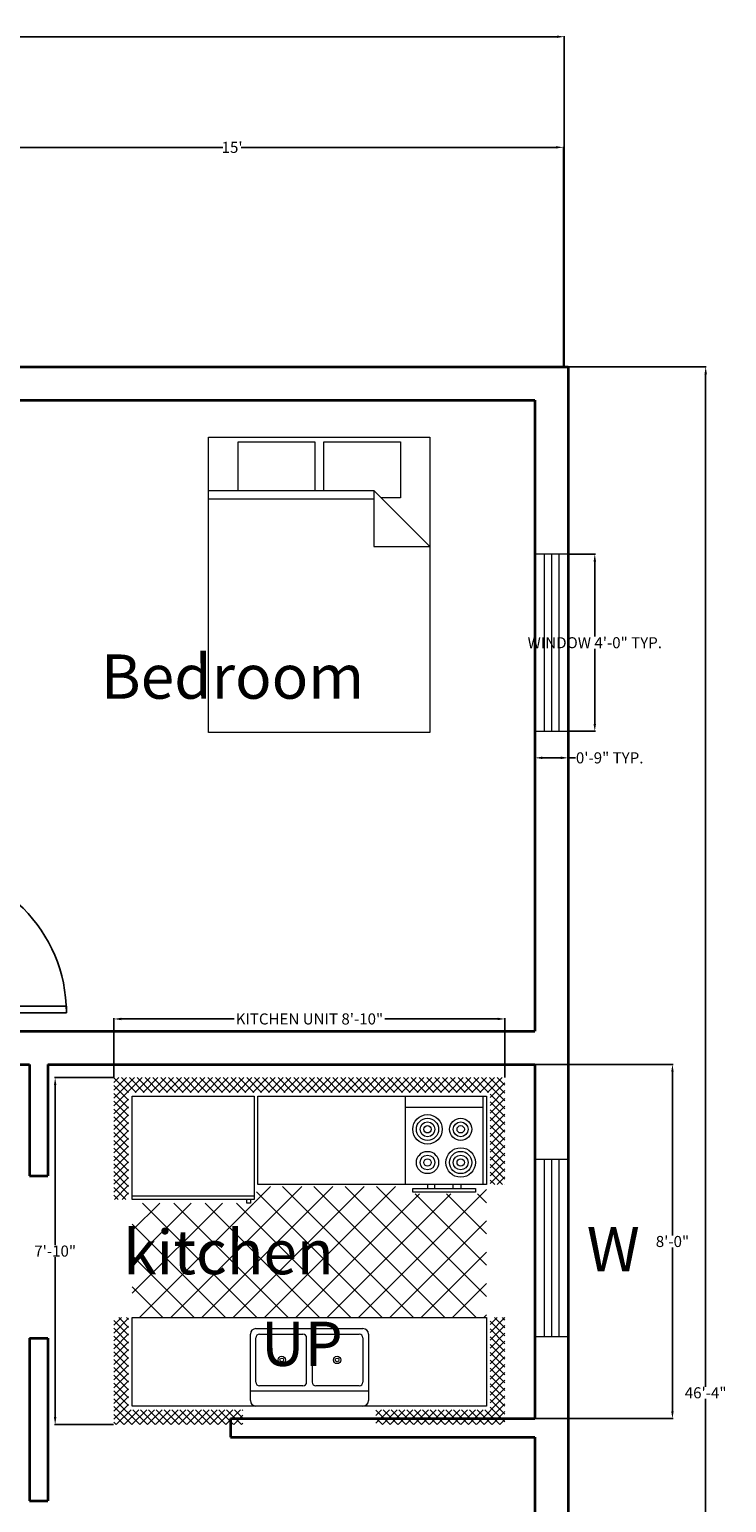
# Model space of a CAD drawing. Units: inches. Extents: x 751 to 1500, y 610 to 1297.
# Tile 4 of 4: x 1308 to 1497, y 898 to 1297. Entities that reach past the tile are written whole.
import ezdxf

# ---------------------------------------------------------------- set-up
doc = ezdxf.new("R2010")
doc.units = ezdxf.units.IN
doc.header["$MEASUREMENT"] = 0
doc.layers.get('0').update_dxf_attribs({"color": 1})
for name, color, linetype, lineweight in [('A-ANNO-DIMS', 5, 'Continuous', 18), ('A-ANNO-TEXT', 7, 'Continuous', 18), ('A-AREA-IDEN', 7, 'Continuous', 25), ('A-FLOR-FIXT', 9, 'Continuous', 18), ('A-FURN', 8, 'Continuous', 18), ('door', 2, 'Continuous', 25), ('wall', 6, 'Continuous', 35), ('windows', 70, 'Continuous', 18)]:
    doc.layers.add(name, color=color, linetype=linetype, lineweight=lineweight)
doc.styles.get("Standard").update_dxf_attribs({"font": 'arial.ttf'})
doc.dimstyles.get("Standard").update_dxf_attribs({"dimtxt": 3, "dimasz": 2, "dimexe": 0.18, "dimexo": 0.0625, "dimgap": 0.09, "dimtad": 0, "dimtih": 1, "dimtoh": 1, "dimdec": 0, "dimzin": 0, "dimdsep": 46, "dimlunit": 3, "dimtxsty": 'Standard', "dimcen": 0.09, "dimadec": 0, "dimazin": 0, "dimtfac": 1, "dimtdec": 0, "dimtofl": 0, "dimtmove": 0, "dimatfit": 3, "dimfxl": 1, "dimtolj": 1, "dimtzin": 0, "dimarcsym": 0})

# ---------------------------------------------------------------- blocks, each defined once
blk = doc.blocks.new('*U3')
for p, q in [((0, 0), (0, 6)), ((40, 0), (40, 6))]:
    blk.add_line(p, q)
blk.add_lwpolyline([(0, 0), (0, -40), (1.75, -40), (1.75, 0)], close=True)
blk.add_arc((0, 0), 40, 270, 360)
blk = doc.blocks.new('*D8')
at = {"layer": 'A-ANNO-DIMS', "color": 0, "lineweight": -2, "transparency": 16777216}
for p, q in [((989.16, 1207.18), (989.16, 1295.32)), ((991.16, 1295.14), (1215.8, 1295.14)), ((1450.93, 1295.14), (1226.29, 1295.14)), ((1452.93, 1205.96), (1452.93, 1295.32))]:
    blk.add_line(p, q, dxfattribs=at)
at = {"layer": 'A-ANNO-DIMS', "color": 0, "transparency": 16777216}
for points in [[(991.16, 1295.48), (991.16, 1294.81), (989.16, 1295.14)], [(1450.93, 1295.48), (1450.93, 1294.81), (1452.93, 1295.14)]]:
    blk.add_solid(points, dxfattribs=at)
at = {"layer": 'Defpoints', "color": 0, "transparency": 16777216}
for p in [(1452.93, 1295.14), (989.16, 1207.12), (1452.93, 1205.9)]:
    blk.add_point(p, dxfattribs=at)
at = {"layer": 'A-ANNO-DIMS', "color": 0, "transparency": 16777216, "insert": (1221.05, 1295.14), "char_height": 3, "attachment_point": 5}
blk.add_mtext('\\A1;38\'-8"', dxfattribs=at)
blk = doc.blocks.new('*D11')
at = {"layer": 'A-ANNO-DIMS', "color": 0, "lineweight": -2, "transparency": 16777216}
for p, q in [((1273.13, 1207.41), (1273.13, 1265.35)), ((1452.66, 1205.46), (1452.66, 1265.35)), ((1275.13, 1265.17), (1360.4, 1265.17)), ((1450.66, 1265.17), (1365.39, 1265.17))]:
    blk.add_line(p, q, dxfattribs=at)
at = {"layer": 'A-ANNO-DIMS', "color": 0, "transparency": 16777216}
for points in [[(1275.13, 1265.51), (1275.13, 1264.84), (1273.13, 1265.17)], [(1450.66, 1265.51), (1450.66, 1264.84), (1452.66, 1265.17)]]:
    blk.add_solid(points, dxfattribs=at)
at = {"layer": 'Defpoints', "color": 0, "transparency": 16777216}
for p in [(1452.66, 1265.17), (1273.13, 1207.34), (1452.66, 1205.4)]:
    blk.add_point(p, dxfattribs=at)
at = {"layer": 'A-ANNO-DIMS', "color": 0, "transparency": 16777216, "insert": (1362.9, 1265.17), "char_height": 3, "attachment_point": 5}
blk.add_mtext("\\A1;15'", dxfattribs=at)
blk = doc.blocks.new('Kitchen Layout - 7 x 8 ft')
for p, q in [((-5, 81.32), (2.68, 89)), ((-5, 83.44), (0.56, 89)), ((-5, 85.56), (-1.56, 89)), ((-5, 87.68), (-3.68, 89)), ((-1, 84.97), (-5, 88.97)), ((1.09, 85), (-2.91, 89)), ((3.21, 85), (-0.79, 89)), ((0.81, 85), (4.81, 89)), ((5.34, 85), (1.34, 89)), ((2.93, 85), (6.93, 89)), ((7.46, 85), (3.46, 89)), ((5.05, 85), (9.05, 89)), ((9.58, 85), (5.58, 89)), ((7.17, 85), (11.17, 89)), ((11.7, 85), (7.7, 89)), ((9.29, 85), (13.29, 89)), ((13.82, 85), (9.82, 89)), ((11.41, 85), (15.41, 89)), ((15.94, 85), (11.94, 89)), ((13.53, 85), (17.53, 89)), ((18.06, 85), (14.06, 89)), ((15.65, 85), (19.65, 89)), ((20.18, 85), (16.18, 89)), ((17.78, 85), (21.78, 89)), ((22.31, 85), (18.31, 89)), ((19.9, 85), (23.9, 89)), ((24.43, 85), (20.43, 89)), ((22.02, 85), (26.02, 89)), ((26.55, 85), (22.55, 89)), ((24.14, 85), (28.14, 89)), ((28.67, 85), (24.67, 89)), ((26.26, 85), (30.26, 89)), ((30.79, 85), (26.79, 89)), ((28.38, 85), (32.38, 89)), ((32.91, 85), (28.91, 89)), ((30.5, 85), (34.5, 89)), ((35.03, 85), (31.03, 89)), ((32.63, 85), (36.63, 89)), ((37.16, 85), (33.16, 89)), ((34.75, 85), (38.75, 89)), ((39.28, 85), (35.28, 89)), ((36.87, 85), (40.87, 89)), ((41.4, 85), (37.4, 89)), ((38.99, 85), (42.99, 89)), ((43.52, 85), (39.52, 89)), ((41.11, 85), (45.11, 89)), ((45.64, 85), (41.64, 89)), ((43.23, 85), (47.23, 89)), ((47.76, 85), (43.76, 89)), ((45.35, 85), (49.35, 89)), ((49.88, 85), (45.88, 89)), ((47.47, 85), (51.47, 89)), ((52, 85), (48, 89)), ((49.6, 85), (53.6, 89)), ((54.13, 85), (50.13, 89)), ((51.72, 85), (55.72, 89)), ((56.25, 85), (52.25, 89)), ((53.84, 85), (57.84, 89)), ((58.37, 85), (54.37, 89)), ((55.96, 85), (59.96, 89)), ((60.49, 85), (56.49, 89)), ((58.08, 85), (62.08, 89)), ((62.61, 85), (58.61, 89)), ((60.2, 85), (64.2, 89)), ((64.73, 85), (60.73, 89)), ((62.32, 85), (66.32, 89)), ((66.85, 85), (62.85, 89)), ((64.45, 85), (68.45, 89)), ((68.97, 85), (64.97, 89)), ((66.57, 85), (70.57, 89)), ((71.1, 85), (67.1, 89)), ((68.69, 85), (72.69, 89)), ((73.22, 85), (69.22, 89)), ((70.81, 85), (74.81, 89)), ((75.34, 85), (71.34, 89)), ((72.93, 85), (76.93, 89)), ((77.46, 85), (73.46, 89)), ((75.05, 85), (79.05, 89)), ((79.58, 85), (75.58, 89)), ((77.17, 85), (81.17, 89)), ((81.7, 85), (77.7, 89)), ((79.29, 85), (83.29, 89)), ((83.82, 85), (79.82, 89)), ((81.42, 85), (85.42, 89)), ((85.95, 85), (81.95, 89)), ((83.54, 85), (87.54, 89)), ((88.07, 85), (84.07, 89)), ((85.66, 85), (89.66, 89)), ((90.19, 85), (86.19, 89)), ((87.78, 85), (91.78, 89)), ((92.31, 85), (88.31, 89)), ((89.9, 85), (93.9, 89)), ((94.43, 85), (90.43, 89)), ((92.02, 85), (96.02, 89)), ((96.55, 85), (92.55, 89)), ((94.14, 85), (98.14, 89)), ((101, 82.67), (94.67, 89)), ((96.27, 85), (100.27, 89)), ((101, 84.79), (96.79, 89)), ((101, 86.92), (98.92, 89)), ((-1, 82.85), (-5, 86.85)), ((-1, 80.73), (-5, 84.73)), ((34, 84), (96, 84)), ((34, 60), (34, 84)), ((96, 84), (96, 60)), ((97, 83.61), (101, 87.61)), ((97, 81.49), (101, 85.49)), ((101, 80.55), (97, 84.55)), ((-5, 79.19), (-1, 83.19)), ((-1, 78.61), (-5, 82.61)), ((-5, 77.07), (-1, 81.07)), ((-1, 76.49), (-5, 80.49)), ((74, 81), (95, 81)), ((97, 79.37), (101, 83.37)), ((101, 78.43), (97, 82.43)), ((97, 77.25), (101, 81.25)), ((101, 76.31), (97, 80.31)), ((-5, 74.95), (-1, 78.95)), ((-1, 74.36), (-5, 78.36)), ((-5, 72.83), (-1, 76.83)), ((-1, 72.24), (-5, 76.24)), ((97, 75.13), (101, 79.13)), ((101, 74.19), (97, 78.19)), ((97, 73.01), (101, 77.01)), ((101, 72.07), (97, 76.07)), ((-5, 70.71), (-1, 74.71)), ((-1, 70.12), (-5, 74.12)), ((-5, 68.59), (-1, 72.59)), ((-1, 68), (-5, 72)), ((97, 70.89), (101, 74.89)), ((101, 69.95), (97, 73.95)), ((97, 68.76), (101, 72.76)), ((-5, 66.47), (-1, 70.47)), ((-1, 65.88), (-5, 69.88)), ((-5, 64.35), (-1, 68.35)), ((101, 67.82), (97, 71.82)), ((97, 66.64), (101, 70.64)), ((101, 65.7), (97, 69.7)), ((97, 64.52), (101, 68.52)), ((-1, 63.76), (-5, 67.76)), ((-5, 62.22), (-1, 66.22)), ((-1, 61.64), (-5, 65.64)), ((-5, 60.1), (-1, 64.1)), ((101, 63.58), (97, 67.58)), ((97, 62.4), (101, 66.4)), ((101, 61.46), (97, 65.46)), ((97, 60.28), (101, 64.28)), ((-1, 59.52), (-5, 63.52)), ((-5, 57.98), (-1, 61.98)), ((-1, 57.39), (-5, 61.39)), ((96, 60), (34, 60)), ((80, 60), (80, 59)), ((82, 59), (82, 60)), ((87, 59), (87, 60)), ((89, 60), (89, 59)), ((100.34, 60), (97, 63.34)), ((98.22, 60), (97, 61.22)), ((98.84, 60), (101, 62.16)), ((100.96, 60), (101, 60.04)), ((-1.73, 56), (-5, 59.27)), ((-3.85, 56), (-5, 57.15)), ((-4.86, 56), (-1, 59.86)), ((-2.74, 56), (-1, 57.74)), ((0, 57), (33, 57)), ((10.4, 24), (45.9, 59.5)), ((18.88, 24), (54.38, 59.5)), ((27.37, 24), (62.87, 59.5)), ((31, 55), (31, 56)), ((32, 56), (32, 55)), ((33.03, 55.11), (37.41, 59.5)), ((67.71, 24), (33.68, 58.04)), ((35.85, 24), (71.35, 59.5)), ((76.2, 24), (40.7, 59.5)), ((44.34, 24), (77.84, 57.5)), ((84.68, 24), (49.18, 59.5)), ((52.82, 24), (86.32, 57.5)), ((93.17, 24), (57.67, 59.5)), ((61.31, 24), (96, 58.69)), ((96, 29.65), (66.15, 59.5)), ((96, 38.14), (76.64, 57.5)), ((96, 46.63), (85.13, 57.5)), ((96, 55.11), (93.57, 57.54)), ((0, 30.57), (24.43, 55)), ((0, 39.06), (15.94, 55)), ((0, 47.54), (7.46, 55)), ((1.91, 24), (32.91, 55)), ((33.77, 24), (2.77, 55)), ((42.26, 24), (11.26, 55)), ((50.74, 24), (19.74, 55)), ((59.23, 24), (28.23, 55)), ((32, 55), (31, 55)), ((25.29, 24), (0, 49.29)), ((69.79, 24), (96, 50.21)), ((16.8, 24), (0, 40.8)), ((78.28, 24), (96, 41.72)), ((8.32, 24), (0, 32.32)), ((86.76, 24), (96, 33.24)), ((-5, 21.92), (-2.92, 24)), ((-1, 21.33), (-3.67, 24)), ((-1, 23.45), (-1.55, 24)), ((0, 24), (96, 24)), ((0, 0), (0, 24)), ((95.25, 24), (96, 24.75)), ((96, 24), (96, 0)), ((97, 22.1), (98.9, 24)), ((97, 19.97), (101, 23.97)), ((101, 21.16), (98.16, 24)), ((101, 23.28), (100.28, 24)), ((-5, 19.8), (-1, 23.8)), ((-1, 19.21), (-5, 23.21)), ((-5, 17.68), (-1, 21.68)), ((-1, 17.09), (-5, 21.09)), ((101, 19.03), (97, 23.03)), ((97, 17.85), (101, 21.85)), ((101, 16.91), (97, 20.91)), ((-5, 15.55), (-1, 19.55)), ((-1, 14.97), (-5, 18.97)), ((-5, 13.43), (-1, 17.43)), ((-1, 12.85), (-5, 16.85)), ((47.25, 6.5), (47.25, 18.5)), ((48.75, 18.5), (48.75, 6.5)), ((97, 15.73), (101, 19.73)), ((101, 14.79), (97, 18.79)), ((97, 13.61), (101, 17.61)), ((101, 12.67), (97, 16.67)), ((-5, 11.31), (-1, 15.31)), ((-1, 10.73), (-5, 14.73)), ((-5, 9.19), (-1, 13.19)), ((-1, 8.6), (-5, 12.6)), ((97, 11.49), (101, 15.49)), ((101, 10.55), (97, 14.55)), ((97, 9.37), (101, 13.37)), ((101, 8.43), (97, 12.43)), ((-5, 7.07), (-1, 11.07)), ((-1, 6.48), (-5, 10.48)), ((-5, 4.95), (-1, 8.95)), ((-1, 4.36), (-5, 8.36)), ((97, 7.25), (101, 11.25)), ((101, 6.31), (97, 10.31)), ((97, 5.12), (101, 9.12)), ((101, 4.18), (97, 8.18)), ((-5, 2.83), (-1, 6.83)), ((-1, 2.24), (-5, 6.24)), ((-5, 0.71), (-1, 4.71)), ((-1, 0.12), (-5, 4.12)), ((64, 4), (32, 4)), ((97, 3), (101, 7)), ((101, 2.06), (97, 6.06)), ((97, 0.88), (101, 4.88)), ((-5, -1.42), (-1, 2.58)), ((2, -5), (-5, 2)), ((-5, -3.54), (-1, 0.46)), ((96, 0), (0, 0)), ((93.24, -5), (101, 2.76)), ((95.36, -5), (101, 0.64)), ((101, -0.06), (97, 3.94)), ((101, -2.18), (97, 1.82)), ((-0.12, -5), (-5, -0.12)), ((-2.25, -5), (-5, -2.25)), ((-4.34, -5), (-0.34, -1)), ((-2.22, -5), (1.78, -1)), ((-0.1, -5), (3.9, -1)), ((4.12, -5), (0.12, -1)), ((2.02, -5), (6.02, -1)), ((6.24, -5), (2.24, -1)), ((4.14, -5), (8.14, -1)), ((8.36, -5), (4.36, -1)), ((6.27, -5), (10.27, -1)), ((10.48, -5), (6.48, -1)), ((8.39, -5), (12.39, -1)), ((12.6, -5), (8.6, -1)), ((10.51, -5), (14.51, -1)), ((14.73, -5), (10.73, -1)), ((12.63, -5), (16.63, -1)), ((16.85, -5), (12.85, -1)), ((14.75, -5), (18.75, -1)), ((18.97, -5), (14.97, -1)), ((16.87, -5), (20.87, -1)), ((21.09, -5), (17.09, -1)), ((18.99, -5), (22.99, -1)), ((23.21, -5), (19.21, -1)), ((21.11, -5), (25.11, -1)), ((25.33, -5), (21.33, -1)), ((23.24, -5), (27.24, -1)), ((27.45, -5), (23.45, -1)), ((25.36, -5), (29.36, -1)), ((29.57, -5), (25.57, -1)), ((27.48, -5), (30, -2.48)), ((30, -3.3), (27.7, -1)), ((30, -1.18), (29.82, -1)), ((66, -2.54), (67.54, -1)), ((66, -4.66), (69.66, -1)), ((69.88, -5), (66, -1.12)), ((67.76, -5), (66, -3.24)), ((67.78, -5), (71.78, -1)), ((72, -5), (68, -1)), ((69.9, -5), (73.9, -1)), ((74.12, -5), (70.12, -1)), ((72.03, -5), (76.03, -1)), ((76.24, -5), (72.24, -1)), ((74.15, -5), (78.15, -1)), ((78.36, -5), (74.36, -1)), ((76.27, -5), (80.27, -1)), ((80.49, -5), (76.49, -1)), ((78.39, -5), (82.39, -1)), ((82.61, -5), (78.61, -1)), ((80.51, -5), (84.51, -1)), ((84.73, -5), (80.73, -1)), ((82.63, -5), (86.63, -1)), ((86.85, -5), (82.85, -1)), ((84.75, -5), (88.75, -1)), ((88.97, -5), (84.97, -1)), ((86.88, -5), (90.88, -1)), ((91.09, -5), (87.09, -1)), ((89, -5), (93, -1)), ((93.21, -5), (89.21, -1)), ((91.12, -5), (95.12, -1)), ((95.34, -5), (91.34, -1)), ((97.46, -5), (93.46, -1)), ((99.58, -5), (95.58, -1)), ((101, -4.3), (97, -0.3)), ((97.48, -5), (101, -1.48)), ((99.6, -5), (101, -3.6)), ((-4.37, -5), (-5, -4.37)), ((29.6, -5), (30, -4.6))]:
    blk.add_line(p, q)
for points in [[(0, 56), (0, 84), (33, 84), (33, 56)], [(74, 60), (74, 84), (95, 84), (95, 60)], [(76, 58), (76, 59), (93, 59), (93, 58)]]:
    blk.add_lwpolyline(points, close=True)
for points in [[(33.5, 21), (62.5, 21)], [(32, 1.5), (32, 19.5)], [(33.5, 6.5), (33.5, 18.5)], [(34.5, 19.5), (46.25, 19.5)], [(49.75, 19.5), (61.5, 19.5)], [(62.5, 18.5), (62.5, 6.5)], [(64, 19.5), (64, 1.5)], [(46.25, 5.5), (34.5, 5.5)], [(61.5, 5.5), (49.75, 5.5)], [(62.5, 0), (33.5, 0)]]:
    blk.add_lwpolyline(points)
for centre, radius in [((80, 75), 4), ((80, 75), 3), ((80, 75), 2), ((80, 75), 1), ((89, 75), 3), ((89, 75), 2), ((89, 75), 1), ((80, 66), 3), ((80, 66), 2), ((89, 66), 4), ((89, 66), 3), ((89, 66), 2), ((80, 66), 1), ((89, 66), 1), ((40.5, 12.5), 1), ((40.5, 12.5), 0.5), ((55.5, 12.5), 1), ((55.5, 12.5), 0.5)]:
    blk.add_circle(centre, radius)
for centre, radius, start, end in [((33.5, 19.5), 1.5, 90, 180), ((62.5, 19.5), 1.5, 0, 90), ((34.5, 18.5), 1, 90, 180), ((46.25, 18.5), 1, 0, 90), ((49.75, 18.5), 1, 90, 180), ((61.5, 18.5), 1, 0, 90), ((34.5, 6.5), 1, 180, 270), ((46.25, 6.5), 1, 270, 0), ((49.75, 6.5), 1, 180, 270), ((61.5, 6.5), 1, 270, 0), ((33.5, 1.5), 1.5, 180, 270), ((62.5, 1.5), 1.5, 270, 0)]:
    blk.add_arc(centre, radius, start, end)
blk = doc.blocks.new('Bed - Queen')
for p, q in [((0, -80.00003), (0, 0)), ((0, 0), (59.99999, 0)), ((59.99999, 0), (59.99999, -80.00003)), ((7.99999, -1.2), (28.79998, -1.2)), ((7.99999, -14.4), (7.99999, -1.2)), ((28.79998, -1.2), (28.79998, -14.4)), ((31.19999, -1.2), (51.99999, -1.2)), ((31.19999, -14.4), (31.19999, -1.2)), ((51.99999, -1.2), (51.99999, -16.4)), ((0, -14.4), (44.8, -14.4)), ((59.99999, -29.6), (44.8, -14.4)), ((44.8, -14.4), (44.8, -29.6)), ((44.8, -16.8), (0, -16.8)), ((51.99999, -16.4), (46.79936, -16.4)), ((44.8, -29.6), (59.99999, -29.6)), ((59.99999, -80.00003), (0, -80.00003))]:
    blk.add_line(p, q)
blk = doc.blocks.new('WIN-48IN-PLAN')
for p, q in [((2.5, 48), (2.5, 0)), ((4.5, 48), (4.5, 0)), ((6.5, 48), (6.5, 0))]:
    blk.add_line(p, q)
blk.add_lwpolyline([(9, 48), (0, 48), (0, 0), (9, 0)], close=True)
blk = doc.blocks.new('*D29')
at = {"layer": 'A-ANNO-DIMS', "color": 0, "lineweight": -2, "transparency": 16777216}
for p, q in [((1454.04, 1154.94), (1461.36, 1154.94)), ((1461.18, 1152.94), (1461.18, 1132.59)), ((1461.18, 1108.94), (1461.18, 1129.3)), ((1454.04, 1106.94), (1461.36, 1106.94))]:
    blk.add_line(p, q, dxfattribs=at)
at = {"layer": 'A-ANNO-DIMS', "color": 0, "transparency": 16777216}
for points in [[(1460.85, 1152.94), (1461.52, 1152.94), (1461.18, 1154.94)], [(1460.85, 1108.94), (1461.52, 1108.94), (1461.18, 1106.94)]]:
    blk.add_solid(points, dxfattribs=at)
at = {"layer": 'Defpoints', "color": 0, "transparency": 16777216}
for p in [(1453.98, 1154.94), (1461.18, 1154.94), (1453.98, 1106.94)]:
    blk.add_point(p, dxfattribs=at)
at = {"layer": 'A-ANNO-DIMS', "color": 0, "transparency": 16777216, "insert": (1461.18, 1130.94), "char_height": 3, "attachment_point": 5}
blk.add_mtext('\\A1;WINDOW 4\'-0" TYP.', dxfattribs=at)
blk = doc.blocks.new('*D30')
at = {"layer": 'A-ANNO-DIMS', "color": 0, "lineweight": -2, "transparency": 16777216}
for p, q in [((1444.98, 1106.88), (1444.98, 1099.56)), ((1453.98, 1106.88), (1453.98, 1099.56)), ((1446.98, 1099.74), (1451.98, 1099.74)), ((1453.98, 1099.74), (1455.98, 1099.74))]:
    blk.add_line(p, q, dxfattribs=at)
at = {"layer": 'A-ANNO-DIMS', "color": 0, "transparency": 16777216}
for points in [[(1446.98, 1100.08), (1446.98, 1099.41), (1444.98, 1099.74)], [(1451.98, 1100.08), (1451.98, 1099.41), (1453.98, 1099.74)]]:
    blk.add_solid(points, dxfattribs=at)
at = {"layer": 'Defpoints', "color": 0, "transparency": 16777216}
for p in [(1444.98, 1106.94), (1453.98, 1106.94), (1453.98, 1099.74)]:
    blk.add_point(p, dxfattribs=at)
at = {"layer": 'A-ANNO-DIMS', "color": 0, "transparency": 16777216, "insert": (1465.22, 1099.74), "char_height": 3, "attachment_point": 5}
blk.add_mtext('\\A1;0\'-9" TYP.', dxfattribs=at)
blk = doc.blocks.new('*D39')
at = {"layer": 'A-ANNO-DIMS', "color": 0, "lineweight": -2, "transparency": 16777216}
for p, q in [((1330.85, 1013.15), (1330.85, 1029.17)), ((1332.85, 1028.99), (1363.42, 1028.99)), ((1434.85, 1028.99), (1404.27, 1028.99)), ((1436.85, 1013.15), (1436.85, 1029.17))]:
    blk.add_line(p, q, dxfattribs=at)
at = {"layer": 'A-ANNO-DIMS', "color": 0, "transparency": 16777216}
for points in [[(1332.85, 1029.32), (1332.85, 1028.65), (1330.85, 1028.99)], [(1434.85, 1029.32), (1434.85, 1028.65), (1436.85, 1028.99)]]:
    blk.add_solid(points, dxfattribs=at)
at = {"layer": 'Defpoints', "color": 0, "transparency": 16777216}
for p in [(1436.85, 1028.99), (1330.85, 1013.09), (1436.85, 1013.09)]:
    blk.add_point(p, dxfattribs=at)
at = {"layer": 'A-ANNO-DIMS', "color": 0, "transparency": 16777216, "insert": (1383.85, 1028.99), "char_height": 3, "attachment_point": 5}
blk.add_mtext('\\A1;KITCHEN UNIT 8\'-10"', dxfattribs=at)
blk = doc.blocks.new('*D40')
at = {"layer": 'A-ANNO-DIMS', "color": 0, "lineweight": -2, "transparency": 16777216}
for p, q in [((1330.79, 1013.09), (1314.77, 1013.09)), ((1314.95, 1011.09), (1314.95, 967.71)), ((1314.95, 921.09), (1314.95, 964.47)), ((1330.79, 919.09), (1314.77, 919.09))]:
    blk.add_line(p, q, dxfattribs=at)
at = {"layer": 'A-ANNO-DIMS', "color": 0, "transparency": 16777216}
for points in [[(1314.61, 1011.09), (1315.28, 1011.09), (1314.95, 1013.09)], [(1314.61, 921.09), (1315.28, 921.09), (1314.95, 919.09)]]:
    blk.add_solid(points, dxfattribs=at)
at = {"layer": 'Defpoints', "color": 0, "transparency": 16777216}
for p in [(1314.95, 1013.09), (1330.85, 1013.09), (1330.85, 919.09)]:
    blk.add_point(p, dxfattribs=at)
at = {"layer": 'A-ANNO-DIMS', "color": 0, "transparency": 16777216, "insert": (1314.95, 966.09), "char_height": 3, "attachment_point": 5}
blk.add_mtext('\\A1;7\'-10"', dxfattribs=at)
blk = doc.blocks.new('*D45')
at = {"layer": 'A-ANNO-DIMS', "color": 0, "lineweight": -2, "transparency": 16777216}
for p, q in [((1454.04, 1205.69), (1491.41, 1205.69)), ((1491.23, 1203.69), (1491.23, 929.31)), ((1491.23, 651.69), (1491.23, 926.07)), ((1454.04, 649.69), (1491.41, 649.69))]:
    blk.add_line(p, q, dxfattribs=at)
at = {"layer": 'A-ANNO-DIMS', "color": 0, "transparency": 16777216}
for points in [[(1490.9, 1203.69), (1491.57, 1203.69), (1491.23, 1205.69)], [(1490.9, 651.69), (1491.57, 651.69), (1491.23, 649.69)]]:
    blk.add_solid(points, dxfattribs=at)
at = {"layer": 'Defpoints', "color": 0, "transparency": 16777216}
for p in [(1453.98, 1205.69), (1491.23, 1205.69), (1453.98, 649.69)]:
    blk.add_point(p, dxfattribs=at)
at = {"layer": 'A-ANNO-DIMS', "color": 0, "transparency": 16777216, "insert": (1491.23, 927.69), "char_height": 3, "attachment_point": 5}
blk.add_mtext('\\A1;46\'-4"', dxfattribs=at)
blk = doc.blocks.new('*D51')
at = {"layer": 'A-ANNO-DIMS', "color": 0, "lineweight": -2, "transparency": 16777216}
for p, q in [((1445.04, 1016.69), (1482.41, 1016.69)), ((1482.23, 1014.69), (1482.23, 970.31)), ((1482.23, 922.69), (1482.23, 967.07)), ((1445.04, 920.69), (1482.41, 920.69))]:
    blk.add_line(p, q, dxfattribs=at)
at = {"layer": 'A-ANNO-DIMS', "color": 0, "transparency": 16777216}
for points in [[(1481.9, 1014.69), (1482.57, 1014.69), (1482.23, 1016.69)], [(1481.9, 922.69), (1482.57, 922.69), (1482.23, 920.69)]]:
    blk.add_solid(points, dxfattribs=at)
at = {"layer": 'Defpoints', "color": 0, "transparency": 16777216}
for p in [(1444.98, 1016.69), (1444.98, 920.69), (1482.23, 920.69)]:
    blk.add_point(p, dxfattribs=at)
at = {"layer": 'A-ANNO-DIMS', "color": 0, "transparency": 16777216, "insert": (1482.23, 968.69), "char_height": 3, "attachment_point": 5}
blk.add_mtext('\\A1;8\'-0"', dxfattribs=at)

msp = doc.modelspace()

# ---------------------------------------------------------------- linework, layer by layer
at = {"layer": 'wall'}
for p, q in [((1296.98, 1205.69), (1453.98, 1205.69)), ((1453.98, 1205.69), (1453.98, 1048.69)), ((1296.98, 1196.69), (1444.98, 1196.69)), ((1444.98, 1196.69), (1444.98, 1048.69)), ((1444.98, 1048.69), (1444.98, 1025.69)), ((1453.98, 1048.69), (1453.98, 952.69)), ((1271.98, 1025.69), (1444.98, 1025.69)), ((1266.98, 1016.69), (1307.98, 1016.69)), ((1307.98, 1016.69), (1307.98, 986.52)), ((1312.98, 1016.69), (1444.98, 1016.69)), ((1312.98, 1016.69), (1312.98, 986.52)), ((1444.98, 1016.69), (1444.98, 952.69)), ((1307.98, 986.52), (1312.98, 986.52)), ((1444.98, 952.69), (1444.98, 920.69)), ((1453.98, 952.69), (1453.98, 850.69)), ((1307.98, 942.48), (1307.98, 898.43)), ((1307.98, 942.48), (1312.98, 942.48)), ((1307.98, 942.48), (1307.98, 898.43)), ((1312.98, 942.48), (1312.98, 920.69)), ((1312.98, 942.48), (1312.98, 898.43)), ((1362.48, 920.69), (1444.98, 920.69)), ((1362.48, 920.69), (1362.48, 915.69)), ((1362.48, 915.69), (1367.98, 915.69)), ((1367.98, 915.69), (1444.98, 915.69)), ((1444.98, 915.69), (1444.98, 850.69)), ((1307.98, 898.43), (1312.98, 898.43))]:
    msp.add_line(p, q, dxfattribs=at)

# ---------------------------------------------------------------- block references
at = {"layer": 'A-FLOR-FIXT'}
msp.add_blockref('Kitchen Layout - 7 x 8 ft', (1335.85, 924.09), dxfattribs=at)
at = {"layer": 'A-FURN'}
msp.add_blockref('Bed - Queen', (1356.52, 1186.61), dxfattribs=at)
at = {"layer": 'door', "rotation": 90}
msp.add_blockref('*U3', (1277.98, 1030.69), dxfattribs=at)
at = {"layer": 'windows'}
for p in [(1444.98, 1106.94), (1444.98, 1106.94), (1444.98, 942.94), (1444.98, 942.94)]:
    msp.add_blockref('WIN-48IN-PLAN', p, dxfattribs=at)

# ---------------------------------------------------------------- texts
at = {"layer": 'A-ANNO-TEXT', "char_height": 12, "attachment_point": 1}
for s, width, insert in [('W', 41.6542, (1459.01, 972.58)), ('UP', 28.1541, (1370.73, 946.97))]:
    msp.add_mtext_dynamic_manual_height_columns(s, width=width, gutter_width=1, heights=[0], dxfattribs=dict(at, insert=insert))
at = {"layer": 'A-AREA-IDEN', "char_height": 12, "attachment_point": 1}
for s, width, insert in [('Bedroom', 61.9104, (1327.37, 1127.76)), ('Bedroom', 61.9104, (1327.37, 1127.76)), ('kitchen', 77.518, (1333.4, 971.81))]:
    msp.add_mtext_dynamic_manual_height_columns(s, width=width, gutter_width=1, heights=[0], dxfattribs=dict(at, insert=insert))

# ---------------------------------------------------------------- dimensions: what is measured, and where the dimension line sits
at = {"layer": 'A-ANNO-DIMS'}
for base, p1, p2, picture, middle in [((1452.93, 1295.14), (989.16, 1207.12), (1452.93, 1205.9), '*D8', (1221.05, 1295.14)), ((1452.66, 1265.17), (1273.13, 1207.34), (1452.66, 1205.4), '*D11', (1362.9, 1265.17))]:
    dim = msp.add_linear_dim(base=base, p1=p1, p2=p2, dimstyle='Standard', override={"dimclrd": 0, "dimclre": 0, "dimclrt": 0}, dxfattribs=at)
    dim.commit()
    dim.dimension.update_dxf_attribs({"geometry": picture, "text_midpoint": middle})
for base, p1, p2, angle, picture, middle in [((1491.23, 1205.69), (1453.98, 649.69), (1453.98, 1205.69), 90, '*D45', (1491.23, 927.69)), ((1482.23, 920.69), (1444.98, 1016.69), (1444.98, 920.69), 270, '*D51', (1482.23, 968.69)), ((1314.95, 1013.09), (1330.85, 919.09), (1330.85, 1013.09), 90, '*D40', (1314.95, 966.09))]:
    dim = msp.add_linear_dim(base=base, p1=p1, p2=p2, angle=angle, dimstyle='Standard', override={"dimdec": 1, "dimlfac": 1, "dimrnd": 0, "dimzin": 1, "dimdsep": 46, "dimlunit": 4, "dimfrac": 2}, dxfattribs=at)
    dim.commit()
    dim.dimension.update_dxf_attribs({"geometry": picture, "text_midpoint": middle})
dim = msp.add_linear_dim(base=(1461.18, 1154.94), p1=(1453.98, 1106.94), p2=(1453.98, 1154.94), angle=90, text='WINDOW <> TYP.', dimstyle='Standard', override={"dimdec": 1, "dimlfac": 1, "dimrnd": 0, "dimzin": 1, "dimdsep": 46, "dimlunit": 4, "dimfrac": 2}, dxfattribs=at)
dim.commit()
dim.dimension.update_dxf_attribs({"geometry": '*D29', "text_midpoint": (1461.18, 1130.94)})
for base, p1, p2, text, picture, middle in [((1453.98, 1099.74), (1444.98, 1106.94), (1453.98, 1106.94), '<> TYP.', '*D30', (1465.22, 1099.74)), ((1436.85, 1028.99), (1330.85, 1013.09), (1436.85, 1013.09), 'KITCHEN UNIT <>', '*D39', (1383.85, 1028.99))]:
    dim = msp.add_linear_dim(base=base, p1=p1, p2=p2, text=text, dimstyle='Standard', override={"dimdec": 1, "dimlfac": 1, "dimrnd": 0, "dimzin": 1, "dimdsep": 46, "dimlunit": 4, "dimfrac": 2}, dxfattribs=at)
    dim.commit()
    dim.dimension.update_dxf_attribs({"geometry": picture, "text_midpoint": middle})

doc.saveas('drawing.dxf')
